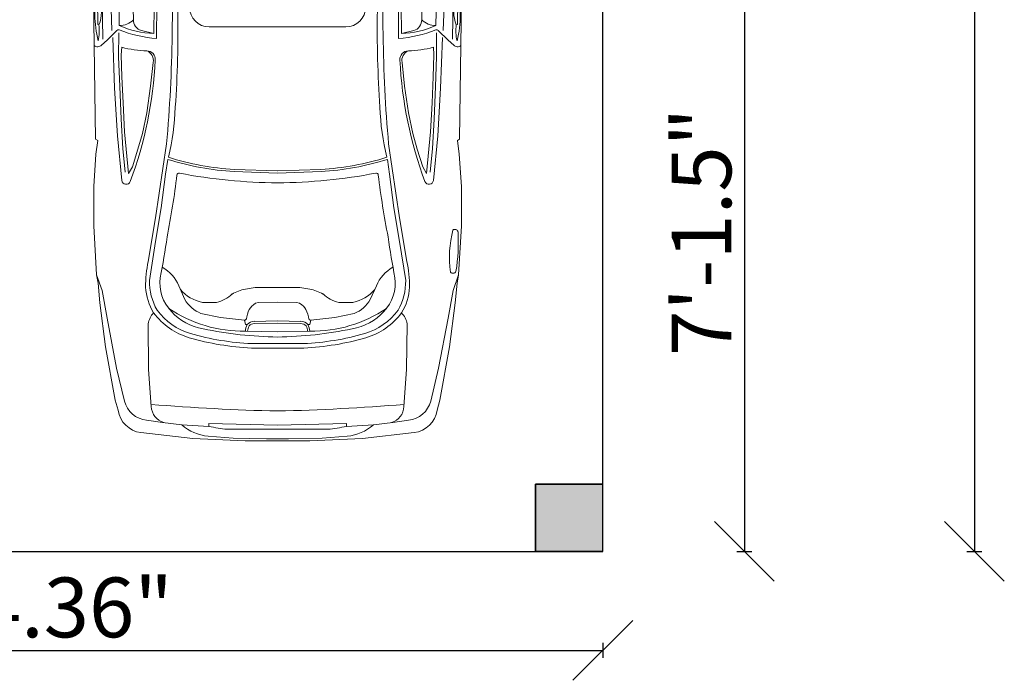
# Model space of a CAD drawing. Units: inches. Extents: x 2561 to 3163, y 493 to 1211.
# Tile 4 of 8: x 3031 to 3163, y 512 to 600. Entities that reach past the tile are written whole.
import ezdxf

# ---------------------------------------------------------------- set-up
doc = ezdxf.new("R2010")
doc.units = ezdxf.units.IN
for name, color, linetype, lineweight in [('0_Equip', 250, 'Continuous', 13), ('A-ANNO-DIMS', 2, 'Continuous', 18), ('A-COLS', 7, 'Continuous', 35), ('A-COLS-PATT', 24, 'Continuous', 13), ('A-SITE-PRKG', 8, 'Continuous', 25)]:
    doc.layers.add(name, color=color, linetype=linetype, lineweight=lineweight)
doc.styles.get("Standard").update_dxf_attribs({"font": 'arial.ttf'})
doc.dimstyles.new('ISO-25', dxfattribs={"dimtxt": 8, "dimasz": 8, "dimexe": 1, "dimexo": 1, "dimtad": 1, "dimlunit": 3, "dimtxsty": 'Standard', "dimblk": 'OBLIQUE', "dimcen": 2.5, "dimadec": 0, "dimazin": 0, "dimtfac": 1, "dimtmove": 0, "dimatfit": 3, "dimfxl": 1, "dimfxlon": 1, "dimarcsym": 0})

# ---------------------------------------------------------------- blocks, each defined once
blk = doc.blocks.new('A$C4C7B54D1')
at = {"layer": '0_Equip', "ltscale": 0.1}
for p, q in [((-1.0176, 2.6505), (-1.112, 2.6343)), ((-0.8531, 2.6707), (-1.0176, 2.6505)), ((-0.7257, 2.678), (-0.8531, 2.6707)), ((-0.7257, 2.678), (-0.5983, 2.6707)), ((-0.5983, 2.6707), (-0.4338, 2.6505)), ((-0.4338, 2.6505), (-0.3394, 2.6343)), ((-1.2037, 2.6168), (-1.3142, 2.5898)), ((-1.1673, 2.6045), (-1.2824, 2.5829)), ((-1.112, 2.6343), (-1.2037, 2.6168)), ((-1.0138, 2.6343), (-1.1673, 2.6045)), ((-0.8877, 2.6027), (-0.9812, 2.5937)), ((-0.8072, 2.6112), (-0.8877, 2.6027)), ((-0.7257, 2.6157), (-0.8072, 2.6112)), ((-0.7257, 2.6157), (-0.6441, 2.6112)), ((-0.6441, 2.6112), (-0.5636, 2.6027)), ((-0.5636, 2.6027), (-0.4701, 2.5937)), ((-0.4376, 2.6343), (-0.284, 2.6045)), ((-0.3394, 2.6343), (-0.2477, 2.6168)), ((-0.284, 2.6045), (-0.1689, 2.5829)), ((-0.2477, 2.6168), (-0.1371, 2.5898)), ((-1.4032, 2.5628), (-1.4801, 2.5318)), ((-1.3789, 2.557), (-1.4667, 2.5181)), ((-1.3142, 2.5898), (-1.4032, 2.5628)), ((-1.2824, 2.5829), (-1.3789, 2.557)), ((-0.1689, 2.5829), (-0.0725, 2.557)), ((-0.1371, 2.5898), (-0.0481, 2.5628)), ((-0.0725, 2.557), (0.0153, 2.5181)), ((-0.0481, 2.5628), (0.0288, 2.5318)), ((-1.4667, 2.5181), (-1.5113, 2.4907)), ((-1.1083, 2.5037), (-1.1486, 2.3827)), ((-0.343, 2.5037), (-0.3027, 2.3827)), ((0.0153, 2.5181), (0.06, 2.4907)), ((-1.5113, 2.4907), (-1.5393, 2.4562)), ((0.06, 2.4907), (0.0879, 2.4562)), ((-1.5353, 2.3701), (-1.5529, 2.308)), ((-1.1486, 2.3827), (-1.1961, 2.1797)), ((-0.3027, 2.3827), (-0.2552, 2.1797)), ((0.084, 2.3701), (0.1016, 2.308)), ((-1.435, 2.1869), (-1.4221, 2.3511)), ((-0.0163, 2.1869), (-0.0293, 2.3511)), ((-1.5529, 2.308), (-1.5677, 2.2486)), ((0.1016, 2.308), (0.1164, 2.2486)), ((-1.5677, 2.2486), (-1.5849, 2.1795)), ((0.1164, 2.2486), (0.1336, 2.1795)), ((-1.597, 2.1976), (-1.615, 2.1169)), ((-1.6012, 2.2082), (-1.597, 2.1976)), ((-1.5849, 2.1795), (-1.5997, 2.1304)), ((-1.4537, 1.863), (-1.435, 2.1869)), ((-1.1961, 2.1797), (-1.2349, 1.9911)), ((-0.2552, 2.1797), (-0.2164, 1.9911)), ((0.0024, 1.863), (-0.0163, 2.1869)), ((0.1336, 2.1795), (0.1484, 2.1304)), ((0.1499, 2.2082), (0.1457, 2.1976)), ((0.1457, 2.1976), (0.1637, 2.1169)), ((-1.5997, 2.1304), (-1.6161, 2.0798)), ((0.1484, 2.1304), (0.1647, 2.0798)), ((-1.615, 2.1169), (-1.6235, 1.8165)), ((0.1637, 2.1169), (0.1722, 1.8165)), ((-1.2349, 1.9911), (-1.2767, 1.8097)), ((-0.2164, 1.9911), (-0.1746, 1.8097)), ((-1.566, 1.8774), (-1.5761, 1.5304)), ((-1.4681, 1.48), (-1.4537, 1.863)), ((0.0168, 1.48), (0.0024, 1.863)), ((0.1147, 1.8774), (0.1247, 1.5304)), ((-1.6235, 1.8165), (-1.6256, 1.5098)), ((-1.2767, 1.8097), (-1.3098, 1.588)), ((-0.1746, 1.8097), (-0.1415, 1.588)), ((0.1722, 1.8165), (0.1743, 1.5098)), ((-1.3098, 1.588), (-1.3443, 1.3187)), ((-0.1415, 1.588), (-0.107, 1.3187)), ((-1.6256, 1.5098), (-1.6129, 1.3846)), ((-1.5761, 1.5304), (-1.5789, 1.1834)), ((0.1247, 1.5304), (0.1276, 1.1834)), ((0.1743, 1.5098), (0.1616, 1.3846)), ((-1.461, 1.1868), (-1.4681, 1.48)), ((-0.955, 1.4459), (-0.955, 1.4827)), ((-0.955, 1.4827), (-0.9321, 1.4827)), ((-0.9321, 1.4827), (-0.9321, 1.4459)), ((-0.5192, 1.4827), (-0.5192, 1.4459)), ((-0.4964, 1.4827), (-0.5192, 1.4827)), ((-0.4964, 1.4459), (-0.4964, 1.4827)), ((0.0097, 1.1868), (0.0168, 1.48)), ((-0.9321, 1.4459), (-0.955, 1.4459)), ((-0.8614, 1.4242), (-0.8603, 1.382)), ((-0.6135, 1.4258), (-0.6012, 1.3814)), ((-0.5809, 1.3459), (-0.5793, 1.4233)), ((-0.5192, 1.4459), (-0.4964, 1.4459)), ((-1.6193, 1.3782), (-1.6252, 0.9375)), ((-1.6129, 1.3846), (-1.6193, 1.3782)), ((-0.8878, 1.3764), (-1.0456, 1.313)), ((-0.7861, 1.3973), (-0.8878, 1.3764)), ((0.1616, 1.3846), (0.1679, 1.3782)), ((0.1679, 1.3782), (0.1739, 0.9375)), ((-0.9361, 1.3119), (-0.8835, 1.3269)), ((-0.8835, 1.3269), (-0.7975, 1.3408)), ((-1.0456, 1.313), (-1.4462, 1.1776)), ((-1.2207, 1.2292), (-1.0263, 1.2883)), ((-1.0263, 1.2883), (-0.9361, 1.3119)), ((-1.4366, 1.1604), (-1.2207, 1.2292)), ((-1.4565, 1.1447), (-1.461, 1.1868)), ((-1.3162, 1.2215), (-1.3088, 1.2011)), ((-1.1723, 1.1976), (-1.2762, 1.1716)), ((-1.0667, 1.22), (-1.1723, 1.1976)), ((-0.3847, 1.22), (-0.279, 1.1976)), ((-0.279, 1.1976), (-0.1751, 1.1716)), ((0.0052, 1.1447), (0.0097, 1.1868)), ((-1.5793, 1.1562), (-1.5793, 0.9761)), ((-1.5552, 1.139), (-1.5552, 0.9693)), ((-1.4503, 1.1151), (-1.4565, 1.1447)), ((-1.4462, 1.1776), (-1.4366, 1.1604)), ((-1.3515, 1.142), (-1.3703, 1.1286)), ((-1.2762, 1.1716), (-1.3515, 1.142)), ((-0.7257, 1.1776), (-0.8858, 1.1725)), ((-0.7257, 1.1776), (-0.5655, 1.1725)), ((-0.1751, 1.1716), (-0.0999, 1.142)), ((-0.0999, 1.142), (-0.0811, 1.1286)), ((-0.0011, 1.1151), (0.0052, 1.1447)), ((0.1038, 1.139), (0.1038, 0.9693)), ((0.128, 1.1562), (0.128, 0.9761)), ((-1.444, 1.0892), (-1.4503, 1.1151)), ((-1.4368, 1.0623), (-1.444, 1.0892)), ((-1.39, 1.0981), (-1.3927, 1.0739)), ((-1.3828, 1.1133), (-1.39, 1.0981)), ((-1.3703, 1.1286), (-1.3828, 1.1133)), ((-0.0811, 1.1286), (-0.0685, 1.1133)), ((-0.0685, 1.1133), (-0.0614, 1.0981)), ((-0.0614, 1.0981), (-0.0587, 1.0739)), ((-0.0145, 1.0623), (-0.0073, 1.0892)), ((-0.0073, 1.0892), (-0.0011, 1.1151)), ((-1.4243, 1.0229), (-1.4368, 1.0623)), ((-1.3927, 1.0739), (-1.3918, 1.0533)), ((-1.3918, 1.0533), (-1.3867, 1.0211)), ((-0.0596, 1.0533), (-0.0646, 1.0211)), ((-0.0587, 1.0739), (-0.0596, 1.0533)), ((-0.027, 1.0229), (-0.0145, 1.0623)), ((-1.5149, 1.011), (-1.4844, 0.9277)), ((-1.4064, 0.961), (-1.4243, 1.0229)), ((-1.3867, 1.0211), (-1.3374, 0.8446)), ((-0.0646, 1.0211), (-0.1139, 0.8446)), ((-0.0449, 0.961), (-0.027, 1.0229)), ((0.0635, 1.011), (0.0331, 0.9277)), ((-1.6252, 0.9375), (-1.5546, 0.9696)), ((-1.3759, 0.8562), (-1.4064, 0.961)), ((-0.0754, 0.8562), (-0.0449, 0.961)), ((0.1739, 0.9375), (0.1032, 0.9696)), ((-1.6745, 0.908), (-1.7088, 0.8764)), ((-1.6252, 0.9375), (-1.6745, 0.908)), ((-1.4844, 0.9277), (-1.4486, 0.8345)), ((0.0331, 0.9277), (-0.0028, 0.8345)), ((0.1739, 0.9375), (0.2232, 0.908)), ((0.2232, 0.908), (0.2574, 0.8764)), ((-1.5321, 0.8786), (-1.7381, 0.7945)), ((-1.5253, 0.865), (-1.7329, 0.7802)), ((-1.7088, 0.8764), (-1.728, 0.8432)), ((-1.5273, 0.8512), (-1.7203, 0.7738)), ((-1.508, 0.8914), (-1.5321, 0.8786)), ((-1.4835, -0.0735), (-1.497, 0.863)), ((-1.3401, 0.7406), (-1.3759, 0.8562)), ((-0.1112, 0.7406), (-0.0754, 0.8562)), ((0.0322, -0.0735), (0.0457, 0.863)), ((0.0566, 0.8914), (0.0807, 0.8786)), ((0.074, 0.865), (0.2816, 0.7802)), ((0.0759, 0.8512), (0.269, 0.7738)), ((0.0807, 0.8786), (0.2867, 0.7945)), ((0.2574, 0.8764), (0.2767, 0.8432)), ((-1.7366, 0.8127), (-1.7377, 0.7934)), ((-1.728, 0.8432), (-1.7366, 0.8127)), ((-1.6171, 0.8152), (-1.5964, -0.6171)), ((-1.5805, 0.8299), (-1.5623, -0.138)), ((-1.5337, 0.8406), (-1.5355, 0.484)), ((-1.4486, 0.8345), (-1.4226, 0.7503)), ((-1.3374, 0.8446), (-1.3097, 0.7577)), ((-0.1139, 0.8446), (-0.1417, 0.7577)), ((-0.0028, 0.8345), (-0.0287, 0.7503)), ((0.0824, 0.8406), (0.0842, 0.484)), ((0.1292, 0.8299), (0.111, -0.138)), ((0.1658, 0.8152), (0.145, -0.6171)), ((0.2767, 0.8432), (0.2853, 0.8127)), ((0.2853, 0.8127), (0.2863, 0.7934)), ((-1.7377, 0.7934), (-1.7327, 0.7794)), ((-1.4352, 0.792), (-1.4152, -0.045)), ((-1.3097, 0.7577), (-1.2953, 0.7129)), ((-0.7257, 0.7541), (-0.7926, 0.7532)), ((-0.7257, 0.7541), (-0.6587, 0.7532)), ((-0.1417, 0.7577), (-0.156, 0.7129)), ((-0.0162, 0.792), (-0.0361, -0.045)), ((0.2863, 0.7934), (0.2813, 0.7794)), ((-1.4226, 0.7503), (-1.4029, 0.6849)), ((-1.315, 0.66), (-1.3401, 0.7406)), ((-1.2953, 0.7129), (-1.2801, 0.6573)), ((-0.7926, 0.7532), (-0.8418, 0.7514)), ((-0.6587, 0.7532), (-0.6095, 0.7514)), ((-0.156, 0.7129), (-0.1712, 0.6573)), ((-0.1363, 0.66), (-0.1112, 0.7406)), ((-0.0287, 0.7503), (-0.0484, 0.6849)), ((-1.4029, 0.6849), (-1.368, 0.5729)), ((-1.2951, 0.5849), (-1.315, 0.66)), ((-0.1562, 0.5849), (-0.1363, 0.66)), ((-0.0484, 0.6849), (-0.0834, 0.5729)), ((-1.2801, 0.6573), (-1.2795, 0.6546)), ((-1.2021, 0.6133), (-1.2663, 0.5956)), ((-1.1177, 0.6302), (-1.2021, 0.6133)), ((-1.0437, 0.6403), (-1.1177, 0.6302)), ((-1.0411, 0.6196), (-1.1142, 0.6096)), ((-0.9389, 0.6526), (-1.0437, 0.6403)), ((-0.937, 0.6317), (-1.0411, 0.6196)), ((-0.8346, 0.6593), (-0.9389, 0.6526)), ((-0.834, 0.6384), (-0.937, 0.6317)), ((-0.7257, 0.6582), (-0.8346, 0.6593)), ((-0.7257, 0.6373), (-0.834, 0.6384)), ((-0.7257, 0.6582), (-0.6168, 0.6593)), ((-0.7257, 0.6373), (-0.6173, 0.6384)), ((-0.6173, 0.6384), (-0.5143, 0.6317)), ((-0.6168, 0.6593), (-0.5124, 0.6526)), ((-0.5143, 0.6317), (-0.4102, 0.6196)), ((-0.5124, 0.6526), (-0.4076, 0.6403)), ((-0.4102, 0.6196), (-0.3371, 0.6096)), ((-0.4076, 0.6403), (-0.3337, 0.6302)), ((-0.3337, 0.6302), (-0.2492, 0.6133)), ((-0.2492, 0.6133), (-0.185, 0.5956)), ((-0.1712, 0.6573), (-0.1719, 0.6546)), ((-1.368, 0.5729), (-1.3527, 0.5066)), ((-1.2663, 0.5956), (-1.2951, 0.5849)), ((-1.2879, 0.5653), (-1.2951, 0.5849)), ((-1.2599, 0.5757), (-1.2879, 0.5653)), ((-1.1973, 0.593), (-1.2599, 0.5757)), ((-1.1142, 0.6096), (-1.1973, 0.593)), ((-0.3371, 0.6096), (-0.2541, 0.593)), ((-0.2541, 0.593), (-0.1914, 0.5757)), ((-0.1914, 0.5757), (-0.1635, 0.5653)), ((-0.185, 0.5956), (-0.1562, 0.5849)), ((-0.1635, 0.5653), (-0.1562, 0.5849)), ((-0.0834, 0.5729), (-0.0986, 0.5066)), ((-1.5355, 0.484), (-1.5292, 0.2045)), ((-1.3527, 0.5066), (-1.3411, 0.4394)), ((-0.0986, 0.5066), (-0.1102, 0.4394)), ((0.0842, 0.484), (0.0779, 0.2045)), ((-1.3411, 0.4394), (-1.3321, 0.3749)), ((-0.1102, 0.4394), (-0.1192, 0.3749)), ((-0.7257, 0.4085), (-1.0528, 0.4085)), ((-0.7257, 0.4085), (-0.3986, 0.4085)), ((-1.3321, 0.3749), (-1.3286, 0.3301)), ((-1.3286, 0.3301), (-1.3204, 0.1751)), ((-1.3178, 0.3418), (-1.31, 0.2426)), ((-0.1335, 0.3418), (-0.1413, 0.2426)), ((-0.1228, 0.3301), (-0.1309, 0.1751)), ((-0.1192, 0.3749), (-0.1228, 0.3301)), ((-1.1468, 0.3145), (-1.1468, 0.0145)), ((-0.3045, 0.3145), (-0.3045, 0.0145)), ((-1.31, 0.2426), (-1.306, 0.1454)), ((-0.1413, 0.2426), (-0.1454, 0.1454)), ((-1.5292, 0.2045), (-1.5185, -0.0974)), ((0.0779, 0.2045), (0.0672, -0.0974)), ((-1.3204, 0.1751), (-1.3164, 0.0193)), ((-1.306, 0.1454), (-1.3036, 0.0305)), ((-0.1454, 0.1454), (-0.1478, 0.0305)), ((-0.1309, 0.1751), (-0.1349, 0.0193)), ((-1.5798, 0.0505), (-1.5879, 0.0456)), ((0.1285, 0.0505), (0.1365, 0.0456)), ((-1.5879, 0.0456), (-1.5863, -0.0676)), ((-1.3164, 0.0193), (-1.3178, -0.1112)), ((-1.3036, 0.0305), (-1.3044, -0.1358)), ((-0.1478, 0.0305), (-0.147, -0.1358)), ((-0.1349, 0.0193), (-0.1335, -0.1112)), ((0.1365, 0.0456), (0.1349, -0.0676)), ((-1.5863, -0.0676), (-1.5806, -0.0692)), ((-0.7257, -0.0796), (-1.0528, -0.0796)), ((-0.7257, -0.0796), (-0.3986, -0.0796)), ((0.1349, -0.0676), (0.1293, -0.0692)), ((-1.4948, -0.0965), (-1.5413, -0.143)), ((-1.5147, -0.1299), (-1.5058, -0.3725)), ((-1.4857, -0.1082), (-1.4866, -0.2223)), ((-1.3774, -0.0972), (-1.3178, -0.1112)), ((-0.0739, -0.0972), (-0.1335, -0.1112)), ((0.0344, -0.1082), (0.0352, -0.2223)), ((0.0435, -0.0965), (0.0899, -0.143)), ((0.0633, -0.1299), (0.0545, -0.3725)), ((-1.5413, -0.143), (-1.5686, -0.1663)), ((-1.4713, -0.1773), (-1.4737, -0.2127)), ((0.02, -0.1773), (0.0224, -0.2127)), ((0.0899, -0.143), (0.1172, -0.1663)), ((-1.4866, -0.2223), (-1.4809, -0.3653)), ((-1.4737, -0.2127), (-1.4705, -0.3187)), ((0.0224, -0.2127), (0.0192, -0.3187)), ((0.0352, -0.2223), (0.0296, -0.3653)), ((-1.3211, -0.2496), (-1.3332, -0.3629)), ((-0.1302, -0.2496), (-0.1182, -0.3629)), ((-1.4705, -0.3187), (-1.4649, -0.4424)), ((0.0192, -0.3187), (0.0135, -0.4424)), ((-1.5058, -0.3725), (-1.4922, -0.6007)), ((-1.4809, -0.3653), (-1.4745, -0.5203)), ((-1.3332, -0.3629), (-1.3516, -0.4906)), ((-0.1182, -0.3629), (-0.0997, -0.4906)), ((0.0296, -0.3653), (0.0232, -0.5203)), ((0.0545, -0.3725), (0.0408, -0.6007)), ((-1.4649, -0.4424), (-1.4576, -0.5822)), ((0.0135, -0.4424), (0.0063, -0.5822)), ((-1.3516, -0.4906), (-1.3725, -0.5902)), ((-0.0997, -0.4906), (-0.0788, -0.5902)), ((-1.4745, -0.5203), (-1.4665, -0.6617)), ((0.0232, -0.5203), (0.0151, -0.6617)), ((-1.4922, -0.6007), (-1.4712, -0.814)), ((-1.4576, -0.5822), (-1.4384, -0.7806)), ((-1.3725, -0.5902), (-1.3942, -0.6641)), ((-0.0788, -0.5902), (-0.0571, -0.6641)), ((0.0063, -0.5822), (-0.013, -0.7806)), ((0.0408, -0.6007), (0.0198, -0.814)), ((-1.5964, -0.6171), (-1.5863, -0.6228)), ((-1.5863, -0.6228), (-1.5949, -0.6885)), ((-1.3094, -0.9936), (-1.2569, -0.6398)), ((-0.1419, -0.9936), (-0.1944, -0.6398)), ((0.145, -0.6171), (0.1349, -0.6228)), ((0.1349, -0.6228), (0.1436, -0.6885)), ((-1.5949, -0.6885), (-1.605, -0.843)), ((-1.4665, -0.6617), (-1.4552, -0.7742)), ((-1.3942, -0.6641), (-1.4199, -0.7485)), ((-0.0571, -0.6641), (-0.0314, -0.7485)), ((0.0151, -0.6617), (0.0039, -0.7742)), ((0.1436, -0.6885), (0.1537, -0.843)), ((-1.4199, -0.7485), (-1.4384, -0.7806)), ((-1.2616, -0.7846), (-1.2511, -0.7134)), ((-0.1898, -0.7846), (-0.2003, -0.7134)), ((-0.0314, -0.7485), (-0.013, -0.7806)), ((-1.2826, -0.9445), (-1.2616, -0.7846)), ((-0.9336, -0.7717), (-0.7257, -0.7787)), ((-0.9331, -0.7613), (-0.7253, -0.7683)), ((-0.5182, -0.7613), (-0.726, -0.7683)), ((-0.5177, -0.7717), (-0.7257, -0.7787)), ((-0.1688, -0.9445), (-0.1898, -0.7846)), ((-1.605, -0.843), (-1.605, -1.0322)), ((0.1537, -0.843), (0.1537, -1.0322)), ((-1.3094, -1.1068), (-1.2826, -0.9445)), ((-0.1419, -1.1068), (-0.1688, -0.9445)), ((-1.605, -1.0322), (-1.592, -1.2661)), ((-1.3444, -1.2014), (-1.3094, -0.9936)), ((-0.1069, -1.2014), (-0.1419, -0.9936)), ((0.1537, -1.0322), (0.1407, -1.2661)), ((-1.3386, -1.2925), (-1.3094, -1.1068)), ((-0.1127, -1.2925), (-0.1419, -1.1068)), ((-1.565, -1.3405), (-1.592, -1.2661)), ((-1.592, -1.2661), (-1.5848, -1.3051)), ((0.1137, -1.3405), (0.1407, -1.2661)), ((0.1407, -1.2661), (0.1335, -1.3051)), ((-1.5848, -1.3051), (-1.5762, -1.4004)), ((-1.1985, -1.3182), (-1.1694, -1.3835)), ((-0.2528, -1.3182), (-0.282, -1.3835)), ((0.1335, -1.3051), (0.1248, -1.4004)), ((-1.5417, -1.4736), (-1.565, -1.3405)), ((-0.88, -1.3337), (-0.8328, -1.3271)), ((-0.8328, -1.3271), (-0.7257, -1.3271)), ((-0.6185, -1.3271), (-0.7257, -1.3271)), ((-0.5713, -1.3337), (-0.6185, -1.3271)), ((0.0904, -1.4736), (0.1137, -1.3405)), ((-1.5762, -1.4004), (-1.5486, -1.6107)), ((-1.0858, -1.3979), (-1.0181, -1.3979)), ((-0.8409, -1.4088), (-0.8488, -1.4158)), ((-0.8309, -1.402), (-0.8409, -1.4088)), ((-0.8163, -1.3979), (-0.8309, -1.402)), ((-0.7257, -1.3974), (-0.8163, -1.3979)), ((-0.7257, -1.3974), (-0.635, -1.3979)), ((-0.635, -1.3979), (-0.6204, -1.402)), ((-0.6204, -1.402), (-0.6104, -1.4088)), ((-0.6104, -1.4088), (-0.6025, -1.4158)), ((-0.3655, -1.3979), (-0.4333, -1.3979)), ((0.1248, -1.4004), (0.0973, -1.6107)), ((-1.0923, -1.4501), (-0.9989, -1.4699)), ((-0.8696, -1.4545), (-0.8731, -1.467)), ((-0.8664, -1.4423), (-0.8696, -1.4545)), ((-0.861, -1.4312), (-0.8664, -1.4423)), ((-0.8558, -1.4236), (-0.861, -1.4312)), ((-0.8488, -1.4158), (-0.8558, -1.4236)), ((-0.6025, -1.4158), (-0.5955, -1.4236)), ((-0.5955, -1.4236), (-0.5904, -1.4312)), ((-0.5904, -1.4312), (-0.585, -1.4423)), ((-0.585, -1.4423), (-0.5817, -1.4545)), ((-0.5817, -1.4545), (-0.5782, -1.467)), ((-0.359, -1.4501), (-0.4524, -1.4699)), ((-1.4962, -1.7129), (-1.5417, -1.4736)), ((-1.3456, -1.5004), (-1.3433, -1.7188)), ((-0.9989, -1.4699), (-0.8846, -1.4828)), ((-0.8807, -1.4821), (-0.8846, -1.4828)), ((-0.8846, -1.4828), (-0.8799, -1.5038)), ((-0.8769, -1.4791), (-0.8807, -1.4821)), ((-0.8799, -1.5038), (-0.8706, -1.5038)), ((-0.8745, -1.477), (-0.8769, -1.4791)), ((-0.8731, -1.467), (-0.8745, -1.477)), ((-0.7257, -1.4865), (-0.8374, -1.4884)), ((-0.7257, -1.4969), (-0.837, -1.4988)), ((-0.7257, -1.4865), (-0.6139, -1.4884)), ((-0.7257, -1.4969), (-0.6143, -1.4988)), ((-0.5714, -1.5038), (-0.5808, -1.5038)), ((-0.5782, -1.467), (-0.5768, -1.477)), ((-0.5768, -1.477), (-0.5744, -1.4791)), ((-0.5744, -1.4791), (-0.5706, -1.4821)), ((-0.5668, -1.4828), (-0.5714, -1.5038)), ((-0.5706, -1.4821), (-0.5668, -1.4828)), ((-0.4524, -1.4699), (-0.5668, -1.4828)), ((-0.1057, -1.5004), (-0.1081, -1.7188)), ((0.0448, -1.7129), (0.0904, -1.4736)), ((-0.8799, -1.5352), (-0.7257, -1.5393)), ((-0.5714, -1.5352), (-0.7257, -1.5393)), ((-0.8502, -1.5951), (-0.7257, -1.5951)), ((-0.6011, -1.5951), (-0.7257, -1.5951)), ((-1.5486, -1.6107), (-1.5024, -1.8663)), ((-0.8507, -1.616), (-0.7257, -1.616)), ((-0.6006, -1.616), (-0.7257, -1.616)), ((0.0973, -1.6107), (0.0511, -1.8663)), ((-1.4584, -1.8701), (-1.4962, -1.7129)), ((-1.3433, -1.7188), (-1.3304, -1.8962)), ((-0.1081, -1.7188), (-0.1209, -1.8962)), ((0.0071, -1.8701), (0.0448, -1.7129)), ((-1.5024, -1.8663), (-1.4894, -1.914)), ((0.0511, -1.8663), (0.0381, -1.914)), ((-1.2767, -1.9721), (-1.3526, -1.9616)), ((-1.1845, -1.9838), (-1.2767, -1.9721)), ((-1.055, -1.9768), (-1.055, -1.9908)), ((-0.7257, -1.985), (-1.055, -1.9768)), ((-0.7257, -1.985), (-0.3964, -1.9768)), ((-0.3964, -1.9768), (-0.3964, -1.9908)), ((-0.2668, -1.9838), (-0.1746, -1.9721)), ((-0.1746, -1.9721), (-0.0987, -1.9616)), ((-1.3797, -2.0208), (-1.1314, -2.0483)), ((-1.055, -1.9908), (-1.1845, -1.9838)), ((-0.9663, -2.0048), (-0.7257, -2.0048)), ((-0.4851, -2.0048), (-0.7257, -2.0048)), ((-0.3964, -1.9908), (-0.2668, -1.9838)), ((-0.0716, -2.0208), (-0.3199, -2.0483)), ((-1.1314, -2.0483), (-0.8803, -2.0598)), ((-1.0585, -2.0375), (-0.9383, -2.0469)), ((-0.9383, -2.0469), (-0.7784, -2.0504)), ((-0.8803, -2.0598), (-0.7257, -2.0598)), ((-0.7784, -2.0504), (-0.7257, -2.0504)), ((-0.673, -2.0504), (-0.7257, -2.0504)), ((-0.5711, -2.0598), (-0.7257, -2.0598)), ((-0.5131, -2.0469), (-0.673, -2.0504)), ((-0.3199, -2.0483), (-0.5711, -2.0598)), ((-0.3929, -2.0375), (-0.5131, -2.0469))]:
    blk.add_line(p, q, dxfattribs=at)
at = {"layer": '0_Equip'}
for p, q in [((-0.7257, 2.5926), (-0.7905, 2.5897)), ((-0.733, 2.5923), (-0.733, 2.5325)), ((-0.7257, 2.5926), (-0.6608, 2.5897)), ((-0.7183, 2.5923), (-0.7183, 2.5325)), ((-1.0577, 2.5343), (-0.8949, 2.5537)), ((-1.0475, 2.557), (-1.0545, 2.5425)), ((-1.0517, 2.5482), (-0.8949, 2.567)), ((-1.0364, 2.5634), (-1.0475, 2.557)), ((-0.9467, 2.5739), (-1.0364, 2.5634)), ((-0.8628, 2.5838), (-0.9467, 2.5739)), ((-0.8949, 2.567), (-0.8211, 2.5763)), ((-0.8949, 2.5537), (-0.8211, 2.5631)), ((-0.8949, 2.5405), (-0.8211, 2.5498)), ((-0.7905, 2.5897), (-0.8628, 2.5838)), ((-0.8211, 2.5763), (-0.738, 2.5791)), ((-0.8211, 2.5631), (-0.738, 2.5659)), ((-0.8211, 2.5498), (-0.738, 2.5526)), ((-0.738, 2.5791), (-0.733, 2.58)), ((-0.738, 2.5659), (-0.733, 2.5668)), ((-0.738, 2.5526), (-0.733, 2.5536)), ((-0.7133, 2.5791), (-0.7183, 2.58)), ((-0.7133, 2.5659), (-0.7183, 2.5668)), ((-0.7133, 2.5526), (-0.7183, 2.5536)), ((-0.6302, 2.5763), (-0.7133, 2.5791)), ((-0.6302, 2.5631), (-0.7133, 2.5659)), ((-0.6302, 2.5498), (-0.7133, 2.5526)), ((-0.6608, 2.5897), (-0.5886, 2.5838)), ((-0.5564, 2.567), (-0.6302, 2.5763)), ((-0.5564, 2.5537), (-0.6302, 2.5631)), ((-0.5564, 2.5405), (-0.6302, 2.5498)), ((-0.5886, 2.5838), (-0.5046, 2.5739)), ((-0.3996, 2.5482), (-0.5564, 2.567)), ((-0.3936, 2.5343), (-0.5564, 2.5537)), ((-0.5046, 2.5739), (-0.4149, 2.5634)), ((-0.4149, 2.5634), (-0.4038, 2.557)), ((-0.4038, 2.557), (-0.3968, 2.5425)), ((-1.0545, 2.5425), (-1.0638, 2.5185)), ((-1.0638, 2.5185), (-1.0638, 2.5092)), ((-1.0638, 2.5092), (-1.0545, 2.504)), ((-1.0631, 2.5204), (-0.8949, 2.5405)), ((-1.0545, 2.504), (-1.0376, 2.5051)), ((-1.0376, 2.5051), (-1.0067, 2.5116)), ((-1.0067, 2.5116), (-0.9502, 2.5168)), ((-0.9502, 2.5168), (-0.8657, 2.5238)), ((-0.8657, 2.5238), (-0.7922, 2.5308)), ((-0.7922, 2.5308), (-0.7433, 2.5325)), ((-0.7433, 2.5325), (-0.7257, 2.5325)), ((-0.7389, 2.5095), (-0.7395, 2.5059)), ((-0.6947, 2.4974), (-0.7261, 2.4828)), ((-0.708, 2.5325), (-0.7257, 2.5325)), ((-0.6947, 2.4974), (-0.723, 2.4776)), ((-0.7124, 2.5095), (-0.7119, 2.5059)), ((-0.6591, 2.5308), (-0.708, 2.5325)), ((-0.5857, 2.5238), (-0.6591, 2.5308)), ((-0.5011, 2.5168), (-0.5857, 2.5238)), ((-0.3882, 2.5204), (-0.5564, 2.5405)), ((-0.4446, 2.5116), (-0.5011, 2.5168)), ((-0.4137, 2.5051), (-0.4446, 2.5116)), ((-0.3968, 2.504), (-0.4137, 2.5051)), ((-0.3968, 2.5425), (-0.3875, 2.5185)), ((-0.3875, 2.5092), (-0.3968, 2.504)), ((-0.3875, 2.5185), (-0.3875, 2.5092)), ((-0.7566, 2.4971), (-0.7261, 2.4828)), ((-0.7566, 2.4971), (-0.7291, 2.4776)), ((-0.7259, 2.4578), (-0.7291, 2.4776)), ((-0.7259, 2.4578), (-0.723, 2.4776))]:
    blk.add_line(p, q, dxfattribs=at)
at = {"layer": '0_Equip', "ltscale": 0.1}
for centre in [(-1.4513, 0), (0, 0)]:
    blk.add_circle(centre, 0.00662, dxfattribs=at)
for centre, radius, start, end in [((-1.0252, 2.6508), 0.02, 304.7228, 3.5172), ((-0.4261, 2.6508), 0.02, 176.4828, 235.2772), ((-0.9299, 2.2354), 0.3619, 98.1466, 109.2524), ((-0.5214, 2.2354), 0.3619, 70.7476, 81.8534), ((-0.9799, 2.461), 0.1353, 120.8369, 151.2853), ((-0.4714, 2.461), 0.1353, 28.7147, 59.1631), ((-1.4391, 2.4422), 0.0986, 114.5945, 157.5113), ((-1.2153, 2.6098), 0.1432, 299.1564, 328.1831), ((-0.9799, 2.461), 0.1353, 151.2853, 161.5889), ((-1.0728, 2.5126), 0.029, 152.6038, 261.721), ((-0.6679, -0.6671), 3.1773, 91.0415, 97.3969), ((-0.7834, -0.6671), 3.1773, 82.6031, 88.9585), ((-0.3785, 2.5126), 0.029, 278.279, 27.3962), ((-0.236, 2.6098), 0.1432, 211.8169, 240.8436), ((-0.4714, 2.461), 0.1353, 18.4111, 28.7147), ((-0.0123, 2.4422), 0.0986, 22.4887, 65.4055), ((-0.4722, 2.0579), 1.139, 158.2564, 172.4203), ((-1.2841, 2.5028), 0.0501, 260.5448, 306.7068), ((-0.1672, 2.5028), 0.0501, 233.2932, 279.4552), ((-0.9791, 2.0579), 1.139, 7.5797, 21.7436), ((-1.4083, 2.3394), 0.1306, 130.2084, 166.4224), ((-1.4798, 2.4259), 0.0184, 54.8052, 134.0204), ((0.0285, 2.4259), 0.0184, 45.9796, 125.1948), ((-0.043, 2.3394), 0.1306, 13.5776, 49.7916), ((0.5502, 1.746), 1.9445, 161.1117, 170.7019), ((-2.0015, 1.746), 1.9445, 9.2981, 18.8883), ((1.1202, 1.7918), 2.6875, 169.5541, 178.1755), ((-2.5715, 1.7918), 2.6875, 1.8245, 10.4459), ((9.2655, 0.7813), 10.7109, 173.14258, 175.77374), ((-10.7169, 0.7813), 10.7109, 4.22626, 6.85742), ((2.9623, 1.2089), 4.3935, 175.2767, 179.1124), ((-4.4136, 1.2089), 4.3935, 0.8876, 4.7233), ((-0.7686, 0.201), 1.2267, 87.9955, 103.2364), ((-0.3726, 1.0935), 0.5131, 139.3585, 143.6922), ((-0.6528, 1.3354), 0.1211, 130.7679, 145.6911), ((-0.6828, 0.201), 1.2267, 76.7636, 92.0045), ((-0.786, 0.3109), 1.1158, 103.6551, 119.1148), ((-0.9216, 1.3498), 0.0409, 323.4512, 39.0343), ((-0.8494, 1.486), 0.1542, 289.6676, 314.192), ((-0.7554, 1.327), 0.0768, 88.1186, 113.6019), ((-0.7803, 1.3768), 0.0384, 357.9275, 44.3829), ((-0.6872, 1.4869), 0.1241, 243.8649, 311.6638), ((-0.6113, 1.3746), 0.0122, 294.8678, 33.6398), ((-0.6653, 0.3109), 1.1158, 60.8852, 76.3449), ((-0.929, 0.5266), 0.803, 96.22, 121.6991), ((-0.7147, 1.4628), 0.1474, 235.8143, 265.7174), ((-0.741, 1.5272), 0.212, 274.1513, 309.4931), ((-0.617, 0.3882), 0.9584, 77.6919, 87.8428), ((-0.5976, 0.2949), 1.0461, 55.3038, 79.8165), ((-1.1803, 0.9494), 0.3676, 113.8511, 139.7847), ((-0.2711, 0.9494), 0.3676, 40.2153, 66.1489), ((-0.7478, -0.378), 1.6295, 89.2231, 101.2856), ((-0.7036, -0.378), 1.6295, 78.7144, 90.7769), ((-1.6261, 1.102), 0.0813, 40.278, 87.0689), ((-1.2706, 1.0395), 0.2408, 142.2718, 177.7746), ((-0.7356, -0.4312), 1.6538, 89.6554, 111.9286), ((-0.7356, -0.4312), 1.6329, 89.6554, 111.9286), ((-0.7157, -0.4312), 1.6538, 68.0714, 90.3446), ((-0.7157, -0.4312), 1.6329, 68.0714, 90.3446), ((-0.1807, 1.0395), 0.2408, 2.2254, 37.7282), ((0.1747, 1.102), 0.0813, 92.9311, 139.722), ((-2.3477, 0.6968), 0.9076, 22.824, 30.2904), ((-0.85, 0.0855), 1.0875, 91.8892, 118.6013), ((-0.6014, 0.0855), 1.0875, 61.3987, 88.1108), ((0.8964, 0.6968), 0.9076, 149.7096, 157.176), ((-1.3493, 1.0932), 0.0105, 111.9286, 291.9286), ((-0.102, 1.0932), 0.0105, 248.0714, 68.0714), ((-1.4887, 1.0171), 0.0269, 132.3277, 193.1064), ((-6.6059, -0.8606), 5.4408, 15.0904, 20.5451), ((5.1546, -0.8606), 5.4408, 159.4549, 164.9096), ((0.0373, 1.0171), 0.0269, 346.8936, 47.6723), ((-1.5684, 0.9084), 0.0628, 344.3283, 77.2348), ((0.1171, 0.9084), 0.0628, 102.7652, 195.6717), ((-1.5495, 0.8614), 0.0245, 335.4987, 44.5114), ((-1.463, 0.9441), 0.0879, 224.7932, 273.9292), ((-1.4233, 0.9849), 0.1262, 227.8287, 253.081), ((0.0117, 0.9441), 0.0879, 266.0708, 315.2068), ((-0.0281, 0.9849), 0.1262, 286.919, 312.1713), ((0.0982, 0.8614), 0.0245, 135.4886, 204.5013), ((-1.7238, 0.7825), 0.00941, 199.646, 291.8616), ((0.2725, 0.7825), 0.00941, 248.1384, 340.354), ((-0.9515, 0.7495), 0.0737, 286.567, 342.4011), ((-0.8474, 0.7163), 0.0355, 80.937, 162.15), ((-0.6039, 0.7163), 0.0355, 17.85, 99.063), ((-0.4998, 0.7495), 0.0737, 197.5989, 253.433), ((-1.1535, 0.5061), 0.2334, 134.9877, 155.4049), ((-0.7896, -1.2957), 1.9795, 94.0807, 103.2045), ((-0.6617, -1.2957), 1.9795, 76.7955, 85.9193), ((-0.2978, 0.5061), 0.2334, 24.5951, 45.0123), ((-1.249, 0.662), 0.0314, 193.667, 283.2045), ((-0.2023, 0.662), 0.0314, 256.7955, 346.333), ((-2.0025, 0.3511), 0.7759, 4.7259, 16.8296), ((0.5512, 0.3511), 0.7759, 163.1704, 175.2741), ((-2.6334, 0.2371), 1.3197, 4.5498, 13.9797), ((-4.2099, -0.0242), 2.9809, 358.1905, 11.4064), ((2.7585, -0.0242), 2.9809, 168.5936, 181.8095), ((1.1821, 0.2371), 1.3197, 166.0203, 175.4502), ((-1.2324, 0.3484), 0.1397, 106.6168, 134.6647), ((-0.2189, 0.3484), 0.1397, 45.3353, 73.3832), ((-6.5594, -0.126), 5.3575, 1.3159, 5.7952), ((-1.0528, 0.3145), 0.0941, 90, 180), ((-0.3986, 0.3145), 0.0941, 0, 90), ((5.1081, -0.126), 5.3575, 174.2048, 178.6841), ((-1.0944, -0.0222), 0.5055, 165.8807, 194.1193), ((-1.3066, 0.102), 0.2781, 180.1936, 190.6834), ((-1.4634, 0.1296), 0.0534, 245.2796, 326.9469), ((0.0121, 0.1296), 0.0534, 213.0531, 294.7204), ((-0.1448, 0.102), 0.2781, 349.3166, 359.8064), ((-0.3569, -0.0222), 0.5055, 345.8807, 14.1193), ((-1.7275, -0.0084), 0.159, 337.4976, 21.7335), ((0.2762, -0.0084), 0.159, 158.2665, 202.5024), ((-1.0528, 0.0145), 0.0941, 180, 270), ((-0.3986, 0.0145), 0.0941, 270, 0), ((-1.4831, 0.0214), 0.095, 269.7172, 315.6185), ((-1.3634, -0.0473), 0.0519, 177.4537, 254.2676), ((-6.573, -0.0941), 5.3705, 356.0501, 0.9723), ((5.1217, -0.0941), 5.3705, 179.0277, 183.9499), ((-0.0879, -0.0473), 0.0519, 285.7324, 2.5463), ((0.0317, 0.0214), 0.095, 224.3815, 270.2828), ((-1.7817, -0.0969), 0.2029, 346.1346, 7.8419), ((-1.4874, -0.1039), 0.0105, 68.8598, 135.0096), ((-1.2476, 0.5164), 0.6547, 248.8598, 265.0222), ((-1.2968, 0.3651), 0.4767, 246.9385, 267.4714), ((-0.2038, 0.5164), 0.6547, 274.9778, 291.1402), ((-0.1545, 0.3651), 0.4767, 272.5286, 293.0615), ((0.0361, -0.1039), 0.0105, 44.9904, 111.1402), ((0.3303, -0.0969), 0.2029, 172.1581, 193.8654), ((-8.0298, -0.0355), 6.7998, 354.90123, 359.30214), ((6.5785, -0.0355), 6.7998, 180.69786, 185.09877), ((-1.5869, -0.1514), 0.0236, 227.2909, 320.7388), ((-1.3362, 0.3542), 0.5484, 255.7347, 268.4072), ((-0.1152, 0.3542), 0.5484, 271.5928, 284.2653), ((0.1355, -0.1514), 0.0236, 219.2612, 312.7091), ((-1.3699, -0.2402), 0.0497, 349.0381, 68.1064), ((-1.3526, -0.2358), 0.0418, 357.143, 88.4072), ((-0.0988, -0.2358), 0.0418, 91.5928, 182.857), ((-0.0814, -0.2402), 0.0497, 111.8936, 190.9619), ((-3.2483, -0.1412), 1.9399, 339.54, 357.143), ((1.797, -0.1412), 1.9399, 182.857, 200.46), ((-2.454, -0.4173), 1.2396, 346.6558, 357.8401), ((1.0027, -0.4173), 1.2396, 182.1599, 193.3442), ((-0.8588, 0.5276), 1.291, 252.4566, 266.6988), ((-0.5926, 0.5276), 1.291, 273.3012, 287.5434), ((-0.8588, 0.5276), 1.3014, 252.4566, 266.7043), ((-0.5926, 0.5276), 1.3014, 273.2957, 287.5434), ((-5.088, -0.3237), 3.9082, 348.7726, 353.1671), ((-1.1971, -0.7899), 0.0105, 79.1189, 173.1671), ((-0.7142, 1.7227), 2.5481, 259.1189, 269.7413), ((-0.7372, 1.7227), 2.5481, 270.2587, 280.8811), ((-0.2542, -0.7899), 0.0105, 6.8329, 100.8811), ((3.6366, -0.3237), 3.9082, 186.8329, 191.2274), ((-1.4504, -0.812), 0.0209, 185.6259, 339.54), ((-0.001, -0.812), 0.0209, 200.46, 354.3741), ((0.625, -1.1812), 0.5281, 165.7822, 187.813), ((0.1224, -1.0639), 0.0155, 11.61, 127.0083), ((-0.7003, -1.1122), 0.8395, 350.5693, 3.5107), ((-4.7286, -0.6026), 3.5073, 348.8701, 352.1003), ((3.2772, -0.6026), 3.5073, 187.8997, 191.1299), ((-0.8187, -1.3185), 0.5386, 167.4447, 180.7102), ((-0.6326, -1.3185), 0.5386, 359.2898, 12.5553), ((-1.3591, -1.3822), 0.1728, 21.7432, 61.9432), ((-0.0922, -1.3822), 0.1728, 118.0568, 158.2568), ((0.1138, -1.243), 0.0156, 219.7819, 334.4738), ((-1.0611, -1.2979), 0.2775, 178.8811, 209.7062), ((-1.0952, -1.3051), 0.1937, 172.4314, 224.4267), ((-0.3561, -1.3051), 0.1937, 315.5733, 7.5686), ((-0.3902, -1.2979), 0.2775, 330.2938, 1.1189), ((-1.0944, -1.3104), 0.2633, 183.2136, 211.504), ((-1.0482, -1.2146), 0.1871, 220.4031, 258.3959), ((-1.0495, -1.2507), 0.1505, 282.0448, 314.7653), ((-0.8301, -1.5634), 0.235, 102.268, 118.8572), ((-0.6213, -1.5634), 0.235, 61.1428, 77.732), ((-0.4019, -1.2507), 0.1505, 225.2347, 257.9552), ((-0.4032, -1.2146), 0.1871, 281.6041, 319.5969), ((-0.3569, -1.3104), 0.2633, 328.496, 356.7864), ((-1.0421, -1.3141), 0.145, 208.6187, 249.7318), ((-0.4092, -1.3141), 0.145, 290.2682, 331.3813), ((-1.2501, -1.516), 0.0967, 135.2951, 170.7274), ((-1.052, -1.2472), 0.3339, 216.9484, 253.2314), ((-1.052, -1.2472), 0.313, 216.9484, 253.2054), ((-0.8912, -0.9022), 0.6331, 235.8724, 271.0227), ((-1.0459, -1.2776), 0.2487, 221.0065, 261.6946), ((-0.5601, -0.9022), 0.6331, 268.9773, 304.1276), ((-0.4054, -1.2776), 0.2487, 278.3054, 318.9935), ((-0.3993, -1.2472), 0.313, 286.7946, 323.0516), ((-0.3993, -1.2472), 0.3339, 286.7686, 323.0516), ((-0.2012, -1.516), 0.0967, 9.2726, 44.7049), ((-0.8066, -1.54), 0.0735, 150.5285, 176.2825), ((-0.8344, -1.538), 0.0498, 93.4455, 136.5439), ((-0.8344, -1.538), 0.0393, 93.7549, 134.7116), ((-0.6169, -1.538), 0.0393, 45.2884, 86.2451), ((-0.6169, -1.538), 0.0498, 43.4561, 86.5545), ((-0.6447, -1.54), 0.0735, 3.7175, 29.4715), ((-0.7884, -0.3101), 1.2865, 254.0263, 267.246), ((-0.7003, 0.2815), 1.8451, 258.0669, 269.2129), ((-0.8066, -1.54), 0.063, 151.7195, 175.9212), ((-0.751, 0.2815), 1.8451, 270.7871, 281.9331), ((-0.6629, -0.3101), 1.2865, 272.754, 285.9737), ((-0.6447, -1.54), 0.063, 4.0788, 28.2805), ((-0.7884, -0.3101), 1.3074, 254.0198, 267.2681), ((-0.6629, -0.3101), 1.3074, 272.7319, 285.9802), ((-1.3393, -1.8393), 0.123, 194.4986, 263.7836), ((-0.1121, -1.8393), 0.123, 276.2164, 345.5014), ((-1.3628, -1.8937), 0.1282, 189.093, 262.4153), ((-0.5134, 7.9307), 9.8503, 265.23745, 268.76503), ((-1.2452, -1.8915), 0.0853, 183.2055, 252.6405), ((-0.938, 7.9307), 9.8503, 271.23497, 274.76255), ((-0.2061, -1.8915), 0.0853, 287.3595, 356.7945), ((-0.0885, -1.8937), 0.1282, 277.5847, 350.907), ((-1.0413, -1.8225), 0.2157, 228.406, 265.4391), ((-0.896, -1.272), 0.7362, 257.5275, 264.5209), ((-0.5554, -1.272), 0.7362, 275.4791, 282.4725), ((-0.41, -1.8225), 0.2157, 274.5609, 311.594)]:
    blk.add_arc(centre, radius, start, end, dxfattribs=at)
for centre, major_axis, ratio in [((-1.399, 2.4187), (-0.1036, -0.0518), 0.497493), ((-1.2016, 2.4892), (0.0562, 0.0189), 0.759763)]:
    blk.add_ellipse(centre, major_axis=major_axis, ratio=ratio, dxfattribs=at)
at = {"layer": '0_Equip'}
blk.add_ellipse((-0.7253, 2.4812), major_axis=(-0.0426, 0), ratio=0.550187, dxfattribs=at)
at = {"layer": '0_Equip', "ltscale": 0.1, "extrusion": (0, 0, -1)}
for centre, major_axis, ratio in [((-0.2497, 2.4892), (-0.0562, 0.0189), 0.759763), ((-0.0523, 2.4187), (0.1036, -0.0518), 0.497493)]:
    blk.add_ellipse(centre, major_axis=major_axis, ratio=ratio, dxfattribs=at)
at = {"layer": '0_Equip', "ltscale": 0.1}
for points, knots in [([(-1.1548, 2.5048), (-1.1596, 2.5191), (-1.1811, 2.5294), (-1.2283, 2.5198), (-1.248, 2.5001), (-1.2511, 2.4679), (-1.2373, 2.4539), (-1.1922, 2.4512), (-1.1656, 2.4658), (-1.1532, 2.4906), (-1.1526, 2.4983), (-1.1548, 2.5048)], [0, 0, 0, 0, 1.408119, 1.408119, 2.816238, 2.816238, 4.224358, 4.224358, 5.632477, 5.632477, 6.283185, 6.283185, 6.283185, 6.283185]), ([(-0.2965, 2.5048), (-0.2917, 2.5191), (-0.2703, 2.5294), (-0.2231, 2.5198), (-0.2033, 2.5001), (-0.2003, 2.4679), (-0.2141, 2.4539), (-0.2592, 2.4512), (-0.2858, 2.4658), (-0.2981, 2.4906), (-0.2987, 2.4983), (-0.2965, 2.5048)], [0, 0, 0, 0, 1.408119, 1.408119, 2.816238, 2.816238, 4.224358, 4.224358, 5.632477, 5.632477, 6.283185, 6.283185, 6.283185, 6.283185]), ([(-1.4937, 2.3714), (-1.4901, 2.3641), (-1.4809, 2.3581), (-1.4492, 2.3543), (-1.4277, 2.3571), (-1.3679, 2.3771), (-1.3298, 2.404), (-1.2994, 2.4483), (-1.2993, 2.4626), (-1.3171, 2.4801), (-1.3406, 2.4849), (-1.3989, 2.4733), (-1.4323, 2.4577), (-1.4816, 2.4186), (-1.4956, 2.3954), (-1.4959, 2.3774), (-1.4951, 2.3742), (-1.4937, 2.3714)], [0, 0, 0, 0, 0.646556, 0.646556, 1.293113, 1.293113, 2.410172, 2.410172, 3.309931, 3.309931, 4.20969, 4.20969, 5.109449, 5.109449, 6.031285, 6.031285, 6.283185, 6.283185, 6.283185, 6.283185]), ([(0.0424, 2.3714), (0.0388, 2.3641), (0.0295, 2.3581), (-0.0022, 2.3543), (-0.0236, 2.3571), (-0.0834, 2.3771), (-0.1216, 2.404), (-0.152, 2.4483), (-0.152, 2.4626), (-0.1343, 2.4801), (-0.1108, 2.4849), (-0.0524, 2.4733), (-0.019, 2.4577), (0.0303, 2.4186), (0.0443, 2.3954), (0.0445, 2.3774), (0.0438, 2.3742), (0.0424, 2.3714)], [0, 0, 0, 0, 0.646556, 0.646556, 1.293113, 1.293113, 2.410172, 2.410172, 3.309931, 3.309931, 4.20969, 4.20969, 5.109449, 5.109449, 6.031285, 6.031285, 6.283185, 6.283185, 6.283185, 6.283185])]:
    blk.add_open_spline(points, degree=3, knots=knots, dxfattribs=at)
at = {"layer": '0_Equip'}
blk.add_open_spline([(-0.7708, 2.4812), (-0.7708, 2.4725), (-0.7635, 2.4648), (-0.7294, 2.4499), (-0.6897, 2.4563), (-0.6733, 2.4916), (-0.7036, 2.5102), (-0.7526, 2.5051), (-0.7708, 2.4948), (-0.7708, 2.4812)], degree=3, knots=[0, 0, 0, 0, 0.903923, 0.903923, 2.878844, 2.878844, 4.872977, 4.872977, 6.283185, 6.283185, 6.283185, 6.283185], dxfattribs=at)
blk = doc.blocks.new('_Oblique')
at = {"color": 0, "linetype": 'ByBlock', "lineweight": -2}
blk.add_line((-0.5, -0.5), (0.5, 0.5), dxfattribs=at)
blk = doc.blocks.new('*D12')
at = {"layer": 'A-ANNO-DIMS', "color": 0, "lineweight": -2, "transparency": 16777216}
for p, q in [((3127.21, 614.57), (3129.21, 614.57)), ((3128.21, 614.57), (3128.21, 529.07)), ((3127.21, 529.07), (3129.21, 529.07))]:
    blk.add_line(p, q, dxfattribs=at)
at = {"layer": 'Defpoints', "color": 0, "transparency": 16777216}
for p in [(2965.27, 614.57), (2965.27, 529.07), (3128.21, 529.07)]:
    blk.add_point(p, dxfattribs=at)
at = {"layer": 'A-ANNO-DIMS', "color": 0, "lineweight": -2, "transparency": 16777216, "xscale": 8, "yscale": 8, "zscale": 8}
for p, rotation in [((3128.21, 614.57), 90), ((3128.21, 529.07), 270)]:
    blk.add_blockref('_Oblique', p, dxfattribs=dict(at, rotation=rotation))
at = {"layer": 'A-ANNO-DIMS', "color": 0, "transparency": 16777216, "insert": (3123.5, 571.82), "char_height": 8, "attachment_point": 5, "rotation": 90}
blk.add_mtext('7\'-1.5"', dxfattribs=at)
blk = doc.blocks.new('*D13')
at = {"layer": 'A-ANNO-DIMS', "color": 0, "lineweight": -2, "transparency": 16777216}
for p, q in [((3157.99, 1093.07), (3159.99, 1093.07)), ((3158.99, 1093.07), (3158.99, 529.07)), ((3157.99, 529.07), (3159.99, 529.07))]:
    blk.add_line(p, q, dxfattribs=at)
at = {"layer": 'Defpoints', "color": 0, "transparency": 16777216}
for p in [(3109.27, 1093.07), (3109.27, 529.07), (3158.99, 529.07)]:
    blk.add_point(p, dxfattribs=at)
at = {"layer": 'A-ANNO-DIMS', "color": 0, "lineweight": -2, "transparency": 16777216, "xscale": 8, "yscale": 8, "zscale": 8}
for p, rotation in [((3158.99, 1093.07), 90), ((3158.99, 529.07), 270)]:
    blk.add_blockref('_Oblique', p, dxfattribs=dict(at, rotation=rotation))
at = {"layer": 'A-ANNO-DIMS', "color": 0, "transparency": 16777216, "insert": (3154.37, 811.07), "char_height": 8, "attachment_point": 5, "rotation": 90}
blk.add_mtext("47'", dxfattribs=at)
blk = doc.blocks.new('*D14')
at = {"layer": 'A-ANNO-DIMS', "color": 0, "lineweight": -2, "transparency": 16777216}
for p, q in [((2948.92, 516.82), (2948.92, 514.82)), ((3109.27, 516.82), (3109.27, 514.82)), ((2948.92, 515.82), (3109.27, 515.82))]:
    blk.add_line(p, q, dxfattribs=at)
at = {"layer": 'Defpoints', "color": 0, "transparency": 16777216}
for p in [(2948.92, 529.07), (3109.27, 529.07), (3109.27, 515.82)]:
    blk.add_point(p, dxfattribs=at)
at = {"layer": 'A-ANNO-DIMS', "color": 0, "lineweight": -2, "transparency": 16777216, "xscale": 8, "yscale": 8, "zscale": 8, "rotation": 180}
blk.add_blockref('_Oblique', (2948.92, 515.82), dxfattribs=at)
at = {"layer": 'A-ANNO-DIMS', "color": 0, "lineweight": -2, "transparency": 16777216, "xscale": 8, "yscale": 8, "zscale": 8}
blk.add_blockref('_Oblique', (3109.27, 515.82), dxfattribs=at)
at = {"layer": 'A-ANNO-DIMS', "color": 0, "transparency": 16777216, "insert": (3029.1, 520.53), "char_height": 8, "attachment_point": 5}
blk.add_mtext('13\'-4.36"', dxfattribs=at)
blk = doc.blocks.new('*D17')
at = {"layer": 'A-ANNO-DIMS', "color": 0, "lineweight": -2, "transparency": 16777216}
for p, q in [((2571.63, 1093.07), (2569.63, 1093.07)), ((2570.63, 1093.07), (2570.63, 529.07)), ((2571.63, 529.07), (2569.63, 529.07))]:
    blk.add_line(p, q, dxfattribs=at)
at = {"layer": 'Defpoints', "color": 0, "transparency": 16777216}
for p in [(2629.27, 1093.07), (2570.63, 529.07), (3109.27, 529.07)]:
    blk.add_point(p, dxfattribs=at)
at = {"layer": 'A-ANNO-DIMS', "color": 0, "lineweight": -2, "transparency": 16777216, "xscale": 8, "yscale": 8, "zscale": 8}
for p, rotation in [((2570.63, 1093.07), 90), ((2570.63, 529.07), 270)]:
    blk.add_blockref('_Oblique', p, dxfattribs=dict(at, rotation=rotation))
at = {"layer": 'A-ANNO-DIMS', "color": 0, "transparency": 16777216, "insert": (2566, 811.07), "char_height": 8, "attachment_point": 5, "rotation": 90}
blk.add_mtext("47'", dxfattribs=at)
blk = doc.blocks.new('*D20')
at = {"layer": 'A-ANNO-DIMS', "color": 0, "lineweight": -2, "transparency": 16777216}
for p, q in [((3018.58, 676.33), (3016.58, 676.33)), ((3017.58, 543.86), (3017.58, 676.33)), ((3018.58, 543.86), (3016.58, 543.86))]:
    blk.add_line(p, q, dxfattribs=at)
at = {"layer": 'Defpoints', "color": 0, "transparency": 16777216}
for p in [(3017.58, 676.33), (3037.45, 676.33), (3037.45, 543.86)]:
    blk.add_point(p, dxfattribs=at)
at = {"layer": 'A-ANNO-DIMS', "color": 0, "lineweight": -2, "transparency": 16777216, "xscale": 8, "yscale": 8, "zscale": 8}
for p, rotation in [((3017.58, 676.33), 90), ((3017.58, 543.86), 270)]:
    blk.add_blockref('_Oblique', p, dxfattribs=dict(at, rotation=rotation))
at = {"layer": 'A-ANNO-DIMS', "color": 0, "transparency": 16777216, "insert": (3012.82, 610.1), "char_height": 8, "attachment_point": 5, "rotation": 90}
blk.add_mtext('CAR 11\'-0 1/2"', dxfattribs=at)

msp = doc.modelspace()

# ---------------------------------------------------------------- hatches: boundary and pattern name
at = {"layer": 'A-COLS-PATT'}
h = msp.add_hatch(color=256, dxfattribs=at)
h.dxf.hatch_style = 1
h.paths.add_polyline_path([(3109.274, 538.069), (3100.274, 538.069), (3100.274, 529.069), (3109.274, 529.069)])
h.paths.add_polyline_path([(2957.918, 538.069), (2948.918, 538.069), (2948.918, 529.069), (2957.918, 529.069)])

# ---------------------------------------------------------------- linework, layer by layer
at = {"layer": 'A-COLS'}
for p, q in [((3100.274, 529.069), (3100.274, 538.069)), ((3100.274, 538.069), (3109.274, 538.069)), ((3109.274, 529.069), (3100.274, 529.069))]:
    msp.add_line(p, q, dxfattribs=at)
at = {"layer": 'A-SITE-PRKG'}
for p, q in [((3109.274, 529.069), (3109.274, 695.069)), ((2948.918, 529.069), (3109.274, 529.069))]:
    msp.add_line(p, q, dxfattribs=at)

# ---------------------------------------------------------------- block references
at = {"layer": '0_Equip', "xscale": 27.9602461462663, "yscale": 27.9602461462663, "zscale": 27.9602461462663}
msp.add_blockref('A$C4C7B54D1', (3086.047, 601.455), dxfattribs=at)

# ---------------------------------------------------------------- dimensions: what is measured, and where the dimension line sits
at = {"layer": 'A-ANNO-DIMS'}
for base, p1, p2, override, picture, middle in [((2570.627, 529.069), (2629.274, 1093.069), (3109.274, 529.069), {"dimclrd": 0, "dimclre": 0, "dimclrt": 0}, '*D17', (2566.002, 811.069)), ((3158.992, 529.069), (3109.274, 1093.069), (3109.274, 529.069), {"dimclrd": 0, "dimclre": 0, "dimclrt": 0}, '*D13', (3154.367, 811.069)), ((3128.213, 529.069), (2965.274, 614.569), (2965.274, 529.069), {"dimclrd": 0, "dimclre": 0, "dimclrt": 0, "dimtmove": 1}, '*D12', (3123.503, 571.819))]:
    dim = msp.add_linear_dim(base=base, p1=p1, p2=p2, angle=90, dimstyle='ISO-25', override=override, dxfattribs=at)
    dim.commit()
    dim.dimension.update_dxf_attribs({"geometry": picture, "text_midpoint": middle})
dim = msp.add_linear_dim(base=(3017.58, 676.333), p1=(3037.451, 543.862), p2=(3037.451, 676.333), angle=90, text='CAR <>', dimstyle='ISO-25', override={"dimdec": 1, "dimlfac": 1, "dimrnd": 0, "dimzin": 1, "dimdsep": 46, "dimlunit": 4, "dimfrac": 2}, dxfattribs=at)
dim.commit()
dim.dimension.update_dxf_attribs({"geometry": '*D20', "text_midpoint": (3012.819, 610.098)})
dim = msp.add_linear_dim(base=(3109.274, 515.818), p1=(2948.918, 529.069), p2=(3109.274, 529.069), dimstyle='ISO-25', override={"dimclrd": 0, "dimclre": 0, "dimclrt": 0}, dxfattribs=at)
dim.commit()
dim.dimension.update_dxf_attribs({"geometry": '*D14', "text_midpoint": (3029.096, 520.53)})

doc.saveas('drawing.dxf')
